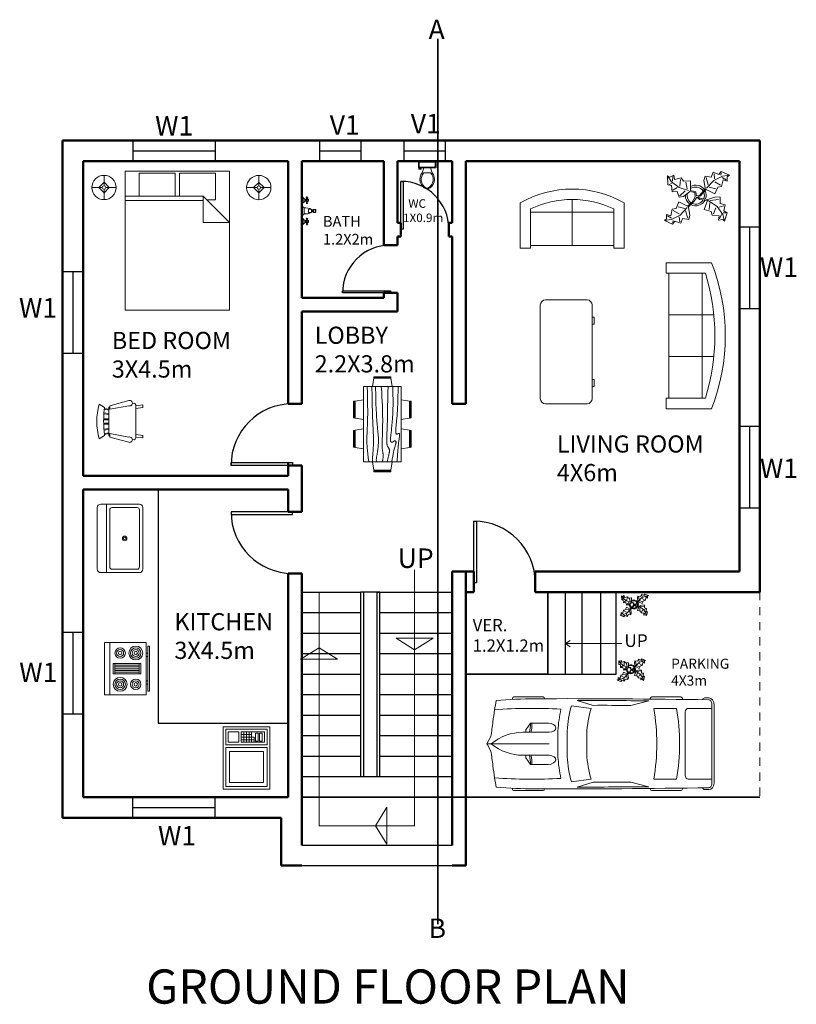
# Paper-space layout 'Layout1' of a CAD drawing. Units: metres. Extents: x 221.2 to 255.5, y 284.4 to 307.4.
# Tile 1 of 3: x 222.2 to 233.6, y 284.4 to 298.8. Entities that reach past the tile are written whole.
import ezdxf

# ---------------------------------------------------------------- set-up
doc = ezdxf.new("R2010")
doc.units = ezdxf.units.M
doc.linetypes.add('ACAD_ISO02W100', pattern=[15, 12, -3])
for name, color, linetype, lineweight in [('A-ANNO-SYMB', 1, 'Continuous', 18), ('A-AREA-IDEN', 11, 'Continuous', 25), ('A-EQPM', 20, 'Continuous', 18), ('A-FLOR-CASE', 20, 'Continuous', 25), ('A-FLOR-FIXT', 20, 'Continuous', 18), ('A-FLOR-PROJ', 7, 'ACAD_ISO02W100', 18), ('A-MODL', 7, 'Continuous', 25), ('A-WALL', 7, 'Continuous', 50), ('car', 150, 'Continuous', 18), ('door', 6, 'Continuous', 25), ('floor', 7, 'Continuous', 35), ('flower', 70, 'Continuous', 18), ('furnitures', 20, 'Continuous', 18), ('section', 1, 'Continuous', 35), ('stair', 2, 'Continuous', 25), ('text', 11, 'Continuous', 25), ('window', 3, 'Continuous', 25)]:
    doc.layers.add(name, color=color, linetype=linetype, lineweight=lineweight)
doc.styles.get("Standard").update_dxf_attribs({"font": 'arial.ttf'})

# ---------------------------------------------------------------- blocks, each defined once
blk = doc.blocks.new('*U21')
for p, q in [((0, 0), (0, -6)), ((40, 0), (40, -6))]:
    blk.add_line(p, q)
blk.add_lwpolyline([(0, 0), (0, 40), (1.75, 40), (1.75, 0)], close=True)
blk.add_arc((0, 0), 40, 0, 90)
blk = doc.blocks.new('*U2')
for p, q in [((0, 0), (0, -6)), ((-40, 0), (-40, -6))]:
    blk.add_line(p, q)
blk.add_lwpolyline([(0, 0), (0, 40), (-1.75, 40), (-1.75, 0)], close=True)
blk.add_arc((0, 0), 40, 90, 180)
blk = doc.blocks.new('Bed - Queen')
for p, q in [((0, -80.00003), (0, 0)), ((0, 0), (59.99999, 0)), ((59.99999, 0), (59.99999, -80.00003)), ((7.99999, -1.2), (28.79998, -1.2)), ((7.99999, -14.4), (7.99999, -1.2)), ((28.79998, -1.2), (28.79998, -14.4)), ((31.19999, -1.2), (51.99999, -1.2)), ((31.19999, -14.4), (31.19999, -1.2)), ((51.99999, -1.2), (51.99999, -16.4)), ((0, -14.4), (44.8, -14.4)), ((44.8, -16.8), (0, -16.8)), ((59.99999, -29.6), (44.8, -14.4)), ((44.8, -14.4), (44.8, -29.6)), ((51.99999, -16.4), (46.79936, -16.4)), ((44.8, -29.6), (59.99999, -29.6)), ((59.99999, -80.00003), (0, -80.00003))]:
    blk.add_line(p, q)
blk = doc.blocks.new('Chair - Rocking')
for p, q in [((-8, -4.5), (-10, -1.5)), ((-7.5, -4.5), (-7, -7)), ((-6.5, -7), (-7.02225, -4.43)), ((-4.5, -7), (-4.96674, -4.19951)), ((-4, -7), (-4.40532, -4.16272)), ((-1.5, -4.05012), (-1.5, -7)), ((-1, -7), (-1, -4.05012)), ((1, -7), (1, -4.04655)), ((1.5, -4.05012), (1.5, -7)), ((4, -7), (4.40187, -4.18694)), ((4.5, -7), (4.96761, -4.19437)), ((6.5, -7), (7, -4.4057)), ((7.5, -4.5), (7, -7)), ((8, -4.5), (10, -1.5)), ((-9, -7.5), (-12, -18.49999)), ((-7, -7.5), (-9, -7.5)), ((-9, -18.49999), (-7, -7.5)), ((-8.23428, -6.99939), (-8.3093, -7.47958)), ((-8.23041, -7), (8.23915, -7)), ((7, -7.5), (9, -7.5)), ((9, -18.49999), (7, -7.5)), ((8.31071, -7.48854), (8.23449, -7.00073)), ((9, -7.5), (12, -18.49999)), ((-10.36644, -20.64523), (-10.5, -21.49999)), ((-9, -22.49999), (-9.5, -26.49999)), ((0, -22.49999), (-9.5, -22.49999)), ((-8, -26.49999), (-7.5, -22.49999)), ((0, -22.49999), (9.5, -22.49999)), ((8, -26.49999), (7.5, -22.49999)), ((9, -22.49999), (9.5, -26.49999)), ((10.5, -21.49999), (10.3575, -20.58798)), ((-9.5, -26.49999), (-8, -26.49999)), ((9.5, -26.49999), (8, -26.49999))]:
    blk.add_line(p, q)
for centre, radius, start, end in [((0, -34.08333), 34.08333, 72.93847, 107.0615), ((0, -68.25004), 64.25, 93.92211, 97.15267), ((0, -68.25004), 64.25, 82.84733, 93.92211), ((-10.5, -18.99999), 1.58114, 161.5651, 18.43495), ((-9.5, -21.49999), 1, 180, 270), ((10.5, -18.99999), 1.58114, 161.5651, 18.43495), ((9.5, -21.49999), 1, 270, 0)]:
    blk.add_arc(centre, radius, start, end)
blk = doc.blocks.new('Dining Set - 36 x 72 in.')
for p, q in [((-22.2343, 26.00059), (-23.4847, 17.99762)), ((-22.2304, 26), (-5.7608, 26)), ((-22, 27.5), (-22.1562, 26.50042)), ((-5.8416, 26.5), (-22.1534, 26.5)), ((-22, 27.5), (-6, 27.5)), ((-5.8437, 26.49966), (-6, 27.5)), ((-4.5152, 17.99762), (-5.7655, 25.99926)), ((5.7657, 26.00059), (4.5153, 17.99762)), ((5.7696, 26), (22.2392, 26)), ((6, 27.5), (5.8438, 26.50042)), ((22.1584, 26.5), (5.8466, 26.5)), ((6, 27.5), (22, 27.5)), ((22.1563, 26.49966), (22, 27.5)), ((23.4848, 17.99762), (22.2345, 25.99926)), ((-44.0006, 8.23428), (-35.9976, 9.48474)), ((36, 18), (-36, 18)), ((-36, 18), (-36, -18)), ((44.0006, 8.23428), (35.9976, 9.48474)), ((36, -18), (36, 18)), ((-45.5, 8), (-44.5004, 8.15617)), ((-45.5, 8), (-45.5, -8)), ((-44.5, -8.15843), (-44.5, 8.15338)), ((-44, 8.23041), (-44, -8.23915)), ((44, 8.23041), (44, -8.23915)), ((44.5, -8.15843), (44.5, 8.15338)), ((45.5, 8), (44.5005, 8.15617)), ((45.5, 8), (45.5, -8)), ((-44.4997, -8.15631), (-45.5, -8)), ((-35.9976, -9.48476), (-43.9993, -8.2345)), ((35.9976, -9.48476), (43.9993, -8.2345)), ((44.4997, -8.15631), (45.5, -8)), ((-36, -18), (36, -18)), ((-22.2343, -26.0006), (-23.4847, -17.99762)), ((-4.5152, -17.99762), (-5.7655, -25.99928)), ((5.7657, -26.0006), (4.5153, -17.99762)), ((23.4848, -17.99762), (22.2345, -25.99928)), ((-22.2304, -26), (-5.7608, -26)), ((-22, -27.5), (-22.1562, -26.50044)), ((-5.8416, -26.5), (-22.1534, -26.5)), ((-22, -27.5), (-6, -27.5)), ((-5.8437, -26.49967), (-6, -27.5)), ((5.7696, -26), (22.2392, -26)), ((6, -27.5), (5.8438, -26.50044)), ((22.1584, -26.5), (5.8466, -26.5)), ((6, -27.5), (22, -27.5)), ((22.1563, -26.49967), (22, -27.5))]:
    blk.add_line(p, q)
for points in [[(-36, 15), (-31.1772, 14.97754), (-26.8079, 14.91406), (-22.8538, 14.81543), (-19.276, 14.6875), (-16.0362, 14.53613), (-13.0957, 14.36718), (-10.4159, 14.18652), (-7.9583, 14), (-5.6904, 13.81315), (-3.6035, 13.63021), (-1.6954, 13.45508), (0.0365, 13.29166), (1.5945, 13.14388), (2.9811, 13.01562), (4.1988, 12.9108), (5.25, 12.83333), (6.1393, 12.78613), (6.8802, 12.76823), (7.4883, 12.77767), (7.9792, 12.8125), (8.3685, 12.87077), (8.6719, 12.95052), (8.9049, 13.0498), (9.0833, 13.16666), (9.2205, 13.29899), (9.3216, 13.44401), (9.3895, 13.59879), (9.4271, 13.76041), (9.4373, 13.92594), (9.4232, 14.09245), (9.3875, 14.257), (9.3333, 14.41666), (9.2638, 14.56917), (9.1836, 14.71484), (9.0975, 14.85465), (9.0104, 14.98958), (8.9272, 15.1206), (8.8529, 15.2487), (8.7922, 15.37483), (8.75, 15.5), (8.7305, 15.62467), (8.7344, 15.74739), (8.7617, 15.86621), (8.8125, 15.97916), (8.8867, 16.08431), (8.9844, 16.17968), (9.1055, 16.26334), (9.25, 16.33333), (9.4189, 16.38802), (9.6172, 16.42708), (9.8506, 16.45052), (10.125, 16.45833), (10.4463, 16.45052), (10.8203, 16.42708), (11.2529, 16.38802), (11.75, 16.33333), (12.3184, 16.26318), (12.9694, 16.17838), (13.7151, 16.07991), (14.5677, 15.96875), (15.5395, 15.84586), (16.6426, 15.71224), (17.8893, 15.56884), (19.2917, 15.41666), (20.859, 15.25667), (22.5879, 15.08984), (24.4721, 14.91715), (26.5052, 14.73958), (28.6809, 14.5581), (30.9929, 14.3737), (33.4347, 14.18733), (36, 14)], [(-36, 10), (-28.9766, 10.14274), (-23.1725, 10.20442), (-18.4241, 10.19775), (-14.5677, 10.13541), (-11.4399, 10.03011), (-8.877, 9.89453), (-6.7154, 9.74137), (-4.7917, 9.58333), (-2.9698, 9.43082), (-1.2246, 9.28515), (0.4415, 9.14534), (2.026, 9.01041), (3.5266, 8.87939), (4.9408, 8.7513), (6.266, 8.62516), (7.5, 8.5), (8.6411, 8.37549), (9.6914, 8.2539), (10.6538, 8.13818), (11.5312, 8.03125), (12.3267, 7.93603), (13.043, 7.85547), (13.6831, 7.79248), (14.25, 7.75), (14.7471, 7.7303), (15.1797, 7.73307), (15.5537, 7.75732), (15.875, 7.80208), (16.1494, 7.86637), (16.3828, 7.94922), (16.5811, 8.04964), (16.75, 8.16666), (16.8944, 8.29915), (17.0143, 8.44531), (17.1089, 8.60319), (17.1771, 8.77083), (17.218, 8.94629), (17.2305, 9.1276), (17.2137, 9.31282), (17.1667, 9.5), (17.0895, 9.6875), (16.987, 9.875), (16.8649, 10.0625), (16.7292, 10.25), (16.5856, 10.4375), (16.4401, 10.625), (16.2985, 10.8125), (16.1667, 11), (16.05, 11.18733), (15.9518, 11.3737), (15.8752, 11.5581), (15.8229, 11.73958), (15.798, 11.91715), (15.8034, 12.08984), (15.842, 12.25667), (15.9167, 12.41666), (16.0295, 12.56836), (16.1784, 12.70833), (16.3605, 12.83268), (16.5729, 12.9375), (16.8127, 13.01888), (17.0768, 13.07291), (17.3625, 13.0957), (17.6667, 13.08333), (17.9894, 13.03312), (18.3418, 12.94726), (18.7382, 12.82918), (19.1927, 12.68229), (19.7195, 12.51001), (20.3327, 12.31575), (21.0465, 12.10294), (21.875, 11.875), (22.8357, 11.63354), (23.959, 11.37304), (25.2786, 11.08618), (26.8282, 10.76562), (28.6414, 10.40405), (30.752, 9.99414), (33.1936, 9.52856), (36, 9)], [(-36, 5.5), (-30.7157, 5.3348), (-26.069, 5.20963), (-21.9946, 5.11767), (-18.4271, 5.05208), (-15.3009, 5.00602), (-12.5508, 4.97265), (-10.1112, 4.94515), (-7.9167, 4.91666), (-5.909, 4.88167), (-4.0586, 4.83984), (-2.3429, 4.79215), (-0.7396, 4.73958), (0.7739, 4.6831), (2.22, 4.6237), (3.6213, 4.56233), (5, 4.5), (6.373, 4.43782), (7.7344, 4.3776), (9.0723, 4.32129), (10.375, 4.27083), (11.6309, 4.22819), (12.8281, 4.19531), (13.9551, 4.17415), (15, 4.16666), (15.954, 4.17448), (16.819, 4.19791), (17.6001, 4.23698), (18.3021, 4.29166), (18.9299, 4.36198), (19.4883, 4.44791), (19.9823, 4.54948), (20.4167, 4.66666), (20.7969, 4.79899), (21.1302, 4.94401), (21.4245, 5.09879), (21.6875, 5.26041), (21.9271, 5.42594), (22.1511, 5.59245), (22.3672, 5.757), (22.5834, 5.91666), (22.8065, 6.06868), (23.0404, 6.21093), (23.2879, 6.34147), (23.5521, 6.45833), (23.8358, 6.55957), (24.142, 6.64323), (24.4735, 6.70735), (24.8334, 6.75), (25.2235, 6.76969), (25.642, 6.76692), (26.0858, 6.74267), (26.5521, 6.69791), (27.0379, 6.63362), (27.5404, 6.55078), (28.0565, 6.45036), (28.5834, 6.33333), (29.1242, 6.19987), (29.7071, 6.04687), (30.3661, 5.87044), (31.1354, 5.66666), (32.0493, 5.43164), (33.142, 5.16146), (34.4475, 4.85221), (36, 4.5)], [(-36, -1), (-30.7915, -0.6591), (-26.0195, -0.38216), (-21.6519, -0.16284), (-17.6563, 0.00521), (-14.0005, 0.12833), (-10.6523, 0.21289), (-7.5796, 0.26522), (-4.75, 0.29166), (-2.134, 0.29793), (0.2878, 0.28711), (2.5317, 0.26163), (4.6146, 0.22396), (6.5529, 0.17651), (8.3633, 0.12174), (10.0623, 0.06209), (11.6667, 0), (13.1899, -0.06201), (14.6341, -0.1211), (15.9982, -0.17432), (17.2813, -0.21875), (18.4823, -0.25147), (19.6003, -0.26953), (20.6343, -0.27002), (21.5834, -0.25), (22.4481, -0.20768), (23.2357, -0.14584), (23.9549, -0.06836), (24.6146, 0.02083), (25.2235, 0.11784), (25.7904, 0.21875), (26.3241, 0.31966), (26.8334, 0.41666), (27.3265, 0.50618), (27.8099, 0.58593), (28.2894, 0.65397), (28.7709, 0.70833), (29.2601, 0.74707), (29.763, 0.76823), (30.2855, 0.76985), (30.8334, 0.75), (31.4088, 0.70784), (31.9994, 0.64713), (32.589, 0.57275), (33.1615, 0.48958), (33.7008, 0.4025), (34.1908, 0.3164), (34.6153, 0.23616), (34.9584, 0.16666), (35.2099, 0.11165), (35.3848, 0.07031), (35.504, 0.04069), (35.5886, 0.02083), (35.6594, 0.00879), (35.7377, 0.0026), (35.8442, 0.00032), (36, 0)], [(-36, -6.5), (-27.1843, -6.31267), (-20.084, -6.1263), (-14.469, -5.9419), (-10.1094, -5.76042), (-6.7752, -5.58285), (-4.2363, -5.41016), (-2.2629, -5.24333), (-0.625, -5.08334), (0.8708, -4.93099), (2.2715, -4.78646), (3.5872, -4.64974), (4.8281, -4.52084), (6.0046, -4.39974), (7.127, -4.28646), (8.2053, -4.18099), (9.25, -4.08334), (10.2705, -3.99382), (11.2734, -3.91407), (12.2647, -3.84603), (13.25, -3.79167), (14.2354, -3.75293), (15.2266, -3.73177), (16.2295, -3.73015), (17.25, -3.75), (18.2912, -3.79248), (19.3451, -3.85547), (20.4009, -3.93604), (21.4479, -4.03125), (22.4754, -4.13819), (23.4727, -4.25391), (24.4289, -4.37549), (25.3334, -4.5), (26.1785, -4.62492), (26.9694, -4.74935), (27.7145, -4.87281), (28.4219, -4.99479), (29.1, -5.11483), (29.7572, -5.23242), (30.4016, -5.34709), (31.0417, -5.45834), (31.6837, -5.56437), (32.3262, -5.65821), (32.9658, -5.73153), (33.599, -5.77604), (34.2224, -5.78345), (34.8327, -5.74545), (35.4264, -5.65373), (36, -5.5)], [(-36, -10), (-26.4022, -9.81299), (-18.4675, -9.62891), (-11.9839, -9.45069), (-6.7396, -9.28125), (-2.5226, -9.12354), (0.8789, -8.98047), (3.6769, -8.85498), (6.0833, -8.75), (8.2767, -8.66765), (10.3021, -8.60677), (12.1712, -8.56543), (13.8958, -8.54167), (15.4876, -8.53353), (16.9583, -8.53907), (18.3197, -8.55632), (19.5834, -8.58334), (20.7616, -8.61841), (21.8685, -8.66081), (22.9188, -8.71004), (23.9271, -8.76563), (24.9081, -8.82707), (25.8763, -8.89388), (26.8465, -8.96558), (27.8334, -9.04167), (28.8474, -9.12118), (29.8828, -9.20117), (30.93, -9.27824), (31.9792, -9.34896), (33.0205, -9.40991), (34.0443, -9.45768), (35.0407, -9.48885), (36, -9.5)], [(-36, -14.5), (-30.0881, -14.33513), (-25.0332, -14.21224), (-20.7312, -14.12647), (-17.0781, -14.07292), (-13.97, -14.04671), (-11.3027, -14.04297), (-8.9724, -14.05681), (-6.875, -14.08334), (-4.9224, -14.11833), (-3.0905, -14.16016), (-1.3709, -14.20785), (0.2448, -14.26042), (1.7647, -14.3169), (3.1973, -14.3763), (4.5507, -14.43767), (5.8333, -14.5), (7.0554, -14.5621), (8.235, -14.62175), (9.3922, -14.67652), (10.5469, -14.72396), (11.7192, -14.76164), (12.929, -14.78711), (14.1965, -14.79794), (15.5417, -14.79167), (16.9933, -14.76424), (18.6152, -14.70508), (20.4804, -14.60197), (22.6615, -14.44271), (25.2312, -14.21509), (28.2624, -13.9069), (31.8277, -13.50594), (36, -13)]]:
    blk.add_lwpolyline(points)
blk = doc.blocks.new('Plant - Rubber or Philodendron')
for p, q in [((-16.2005, 11.4774), (-13.9899, 8.1064)), ((-16.2005, 11.4774), (-14.8639, 10.7964)), ((-16.0159, 6.3329), (-16.2005, 11.4774)), ((-14.8639, 10.7964), (-12.6195, 11.8975)), ((-12.6195, 11.8975), (-12.1909, 9.4345)), ((8.8871, 10.7908), (9.9809, 13.4933)), ((9.9809, 13.4933), (13.3837, 12.301)), ((10.5828, 12.6946), (10.8893, 9.7953)), ((13.3837, 12.301), (14.68, 13.9039)), ((14.5816, 13.2037), (14.3848, 11.8033)), ((14.68, 13.9039), (19.3848, 11.8146)), ((19.3848, 11.8146), (15.3859, 11.3055)), ((19.3848, 11.8146), (18.1868, 10.9119)), ((-14.0069, 5.8704), (-16.0159, 6.3329)), ((-15.3434, 6.5514), (-13.9984, 6.9884)), ((-13.5868, 2.2894), (-14.0069, 5.8704)), ((-13.9899, 8.1064), (-9.5434, 4.7185)), ((-13.3174, 8.325), (-13.0735, 11.0065)), ((-12.1909, 9.4345), (-8.3829, 10.3)), ((-8.8369, 9.409), (-9.0894, 5.6095)), ((-8.3829, 10.3), (-7.0549, 8.501)), ((-7.0549, 8.501), (-3.0284, 8.6941)), ((-4.8529, 4.012), (-5.7184, 7.82)), ((-3.0284, 8.6941), (-3.0709, 3.1041)), ((4.6914, 8.8812), (5.3859, 11.2828)), ((4.6914, 8.8812), (5.5014, 4.4831)), ((5.3859, 11.2828), (8.8871, 10.7908)), ((5.9878, 10.4842), (7.1971, 6.3869)), ((10.3916, 8.7942), (6.2847, 4.4028)), ((15.3859, 11.3055), (10.3916, 8.7942)), ((14.2977, 6.1031), (10.9934, 7.9956)), ((15.7909, 9.1065), (14.8995, 5.3044)), ((15.2875, 10.6053), (17.5907, 9.2105)), ((18.1925, 8.4119), (15.7909, 9.1065)), ((18.1868, 10.9119), (18.1925, 8.4119)), ((-10.6784, 2.491), (-13.5868, 2.2894)), ((-13.1329, 3.1804), (-10.6614, 4.727)), ((-9.5858, -0.8715), (-10.6784, 2.491)), ((-9.5434, 4.7185), (-4.1917, 2.9888)), ((-9.1318, 0.0195), (-5.9793, 2.9025)), ((-7.1228, -0.443), (-3.5248, 2.2131)), ((-3.5248, 2.2131), (-3.3011, 2.4355)), ((-3.3011, 2.4355), (-0.5306, 1.7947)), ((-3.0709, 3.1041), (0.0797, 2.3163)), ((-0.5306, 1.7947), (-0.2255, -0.5527)), ((-0.5306, 1.7947), (-0.5306, 1.7947)), ((0.0797, 2.3163), (0.4866, -0.031)), ((0.4866, -0.031), (2.1141, 0.2298)), ((2.1141, 0.2298), (5.4346, 3.9146)), ((6.1032, 3.6844), (2.8262, -0.031)), ((5.4346, 3.9146), (5.5014, 4.4831)), ((11.1089, 1.1958), (6.1032, 3.6844)), ((7.7005, 4.8881), (11.5025, 3.9967)), ((12.7005, 4.8994), (11.1089, 1.1958)), ((14.8995, 5.3044), (12.7005, 4.8994)), ((-11.3237, -7.2629), (-9.7321, -3.5593)), ((-9.7321, -3.5593), (-4.7264, -6.0479)), ((-7.1228, -0.443), (-9.5858, -0.8715)), ((-2.019, -3.6148), (-4.7264, -6.0479)), ((-4.0579, -6.2781), (-0.9375, -3.1608)), ((-2.019, -3.6148), (-0.2255, -0.5527)), ((-0.9375, -3.1608), (0.5883, -0.8135)), ((0.5883, -0.8135), (2.2447, -2.0916)), ((2.8262, -0.031), (1.3003, -0.5527)), ((1.3003, -0.5527), (2.4193, -1.4655)), ((2.2447, -2.0916), (6.7108, -2.6626)), ((2.4193, -1.4655), (6.895, -2.1175)), ((4.943, -7.9659), (6.7108, -2.6626)), ((11.6605, -0.5413), (6.895, -2.1175)), ((12.3677, -6.1981), (7.219, -2.6772)), ((8.125, -4.0768), (7.7715, -7.9659)), ((8.3544, -2.7453), (13.1973, -2.1704)), ((11.6605, -0.5413), (14.1354, -0.8948)), ((14.1354, -0.8948), (14.1354, -4.4304)), ((14.1354, -4.4304), (16.9638, -5.1375)), ((16.9638, -5.1375), (16.2567, -8.673)), ((-16.8157, -10.7754), (-14.4141, -11.4699)), ((-16.8101, -13.2754), (-16.8157, -10.7754)), ((-14.4141, -11.4699), (-13.5228, -7.6679)), ((-14.0091, -13.669), (-9.0148, -11.1577)), ((-13.5228, -7.6679), (-11.3237, -7.2629)), ((-12.921, -8.4665), (-9.6166, -10.359)), ((-6.3237, -7.2516), (-10.1257, -6.3602)), ((-9.0148, -11.1577), (-4.9047, -6.8122)), ((-4.611, -12.8477), (-5.8203, -8.7504)), ((-4.1246, -6.8466), (-4.0579, -6.2781)), ((-3.3146, -11.2447), (-4.1246, -6.8466)), ((-3.3146, -11.2447), (-4.0092, -13.6463)), ((8.8321, -9.0266), (4.943, -7.9659)), ((9.5392, -11.1479), (8.8321, -9.0266)), ((13.4283, -11.5015), (9.5392, -11.1479)), ((10.2463, -10.4408), (11.6605, -6.9053)), ((15.5496, -10.7943), (12.3677, -6.1981)), ((16.2567, -5.8446), (13.4283, -6.5517)), ((14.8425, -10.7943), (13.7819, -13.2692)), ((16.6103, -14.6834), (15.5496, -10.7943)), ((17.3174, -9.7337), (15.9032, -9.7337)), ((16.2567, -8.673), (18.0245, -9.7337)), ((18.0245, -9.7337), (16.6103, -14.6834)), ((-18.008, -14.1781), (-16.8101, -13.2754)), ((-18.008, -14.1781), (-14.0091, -13.669)), ((-13.3032, -16.2674), (-18.008, -14.1781)), ((-13.9107, -12.9688), (-16.2139, -11.574)), ((-12.0069, -14.6645), (-13.3032, -16.2674)), ((-13.2048, -15.5672), (-13.008, -14.1668)), ((-8.6042, -15.8568), (-12.0069, -14.6645)), ((-9.206, -15.0581), (-9.5126, -12.1588)), ((-7.5103, -13.1543), (-8.6042, -15.8568)), ((-4.0092, -13.6463), (-7.5103, -13.1543)), ((13.0748, -13.9763), (13.4283, -11.5015)), ((15.5496, -13.6228), (13.0748, -13.9763)), ((16.6103, -14.6834), (15.5496, -13.6228))]:
    blk.add_line(p, q)
for centre, radius, start, end in [((0, 0), 6.1275, 34.37569, 120.1028), ((0.0308, 0.1664), 6, 178.6147, 235.1169), ((0.0308, 0.1664), 5, 168.1647, 238.6725), ((-0.0601, -0.2075), 5.2461, 33.82192, 124.9414), ((-0.2664, 0.1682), 5.2775, 338.4094, 20.03007), ((-0.098, 0.1364), 6.1288, 341.2017, 26.09184), ((-0.0234, 0.3825), 6.1492, 242.5812, 331.2714), ((-0.1102, 0.4886), 5.2883, 247.3711, 327.472)]:
    blk.add_arc(centre, radius, start, end)
blk = doc.blocks.new('Sofa - Roundback 7 ft.')
for p, q in [((-12.00002, -32.4421), (-12.00003, -6.5971)), ((11.99997, -32.4421), (11.99998, -6.5971)), ((-36.000027, -34), (-36.000027, -11.4696)), ((-35.999844, -13.3819), (35.9998, -13.3819)), ((35.99998, -34), (35.99998, -11.4696)), ((-36.000027, -32.4421), (35.99998, -32.4421))]:
    blk.add_line(p, q)
for points in [[(-36.000027, -34), (-42.000027, -34), (-42.000027, -8)], [(41.99998, -8), (41.99998, -34), (35.99998, -34)]]:
    blk.add_lwpolyline(points)
for centre, radius, start, end in [((0, -114.25), 114.25, 68.43141, 111.5686), ((-0.00001, -127.1968), 121.1968, 72.72033, 107.2797)]:
    blk.add_arc(centre, radius, start, end)
blk = doc.blocks.new('Sofa - Roundback Loveseat 5 ft.')
for p, q in [((0, -32.44198), (0, -5.99998)), ((-24, -33.99998), (-24, -11.46958)), ((-23.9998, -13.38178), (23.99986, -13.38178)), ((24.00004, -33.99998), (24.00004, -11.46958)), ((-24, -32.44198), (24.00004, -32.44198))]:
    blk.add_line(p, q)
for points in [[(-24, -33.99998), (-30, -33.99998), (-30, -7.99998)], [(30.00004, -7.99998), (30.00004, -33.99998), (24.00004, -33.99998)]]:
    blk.add_lwpolyline(points)
for centre, radius, start, end in [((0, -60.24998), 60.24998, 60.13715, 119.8628), ((0, -61.38438), 55.38444, 64.32083, 115.6792)]:
    blk.add_arc(centre, radius, start, end)
blk = doc.blocks.new('Desk - 30 x 60 in.')
for p, q in [((-26.999995, 0), (26.999995, 0)), ((-29.999995, -27), (-29.999995, -3)), ((29.999995, -3), (29.999995, -27)), ((26.999995, -30), (-26.999995, -30)), ((-20.000005, -30), (-20.000005, -31)), ((-20.000005, -31), (-16.000005, -31)), ((-16.000005, -31), (-16.000005, -30)), ((15.999995, -31), (15.999995, -30)), ((19.999995, -31), (15.999995, -31)), ((19.999995, -30), (19.999995, -31))]:
    blk.add_line(p, q)
for centre, start, end in [((-26.499995, -3.5), 98.1301, 171.8699), ((26.499995, -3.5), 8.130102, 81.8699), ((-26.499995, -26.5), 188.1301, 261.8699), ((26.499995, -26.5), 278.1301, 351.8699)]:
    blk.add_arc(centre, 3.535534, start, end)
blk = doc.blocks.new('Microwave')
for p, q in [((18, 10), (22, 10)), ((22, 9), (18, 9)), ((18, 8), (22, 8)), ((19, 7), (19, 11)), ((20, 11), (20, 7)), ((21, 7), (21, 11)), ((22, 7), (18, 7)), ((20, 6), (18, 6)), ((19, 6), (19, 7)), ((20, 7), (20, 6))]:
    blk.add_line(p, q)
for points in [[(0, 0), (0, 18), (24, 18), (24, 0)], [(1, 1), (1, 17), (16, 17), (16, 1)], [(2.5, 2.5), (2.5, 15.5), (14.5, 15.5), (14.5, 2.5)], [(17, 1), (17, 17), (23, 17), (23, 1)], [(18, 12), (18, 16), (22, 16), (22, 12)], [(18, 2), (18, 11), (22, 11), (22, 2)], [(18.5, 4.5), (18.5, 5.5), (21.5, 5.5), (21.5, 4.5)], [(18.5, 3), (18.5, 4), (21.5, 4), (21.5, 3)]]:
    blk.add_lwpolyline(points, close=True)
blk = doc.blocks.new('Range-Oven - 30 in top')
for p, q in [((0, -3), (30, -3)), ((12, -6), (18, -6)), ((13, -20), (13, -6)), ((14, -6), (14, -20)), ((15, -20), (15, -6)), ((16, -6), (16, -20)), ((17, -20), (17, -6)), ((18, -20), (12, -20)), ((6, -24), (6, -25)), ((8, -25), (8, -24)), ((22, -25), (22, -24)), ((24, -24), (24, -25))]:
    blk.add_line(p, q)
for points in [[(0, -24), (0, 0), (30, 0), (30, -24)], [(12, -21), (12, -5), (18, -5), (18, -21)], [(2, -26), (2, -25), (28, -25), (28, -26)]]:
    blk.add_lwpolyline(points, close=True)
for centre, radius in [((6, -9), 4), ((6, -9), 3), ((6, -9), 2), ((6, -9), 1), ((24, -9), 3), ((24, -9), 2), ((24, -9), 1), ((6, -18), 3), ((6, -18), 2), ((6, -18), 1), ((24, -18), 4), ((24, -18), 3), ((24, -18), 2), ((24, -18), 1)]:
    blk.add_circle(centre, radius)
blk = doc.blocks.new('Sink-single - 30 in top')
blk.add_line((-15, -3.999996), (15, -3.999996))
for points in [[(-13.5, 0), (13.5, 0)], [(-15, -18.499996), (-15, -1.5)], [(15, -1.5), (15, -18.499996)], [(-13.5, -17.499996), (-13.5, -6.499996)], [(-12.5, -5.499996), (12.5, -5.499996)], [(13.5, -6.499996), (13.5, -17.499996)], [(13.5, -19.999996), (-13.5, -19.999996)], [(12.5, -18.499996), (-12.5, -18.499996)]]:
    blk.add_lwpolyline(points)
for radius in [1, 0.5]:
    blk.add_circle((0, -11.999996), radius)
for centre, radius, start, end in [((-13.5, -1.5), 1.5, 90, 180), ((13.5, -1.5), 1.5, 0, 90), ((-12.5, -6.499996), 1, 90, 180), ((12.5, -6.499996), 1, 0, 90), ((-13.5, -18.499996), 1.5, 180, 270), ((-12.5, -17.499996), 1, 180, 270), ((12.5, -17.499996), 1, 270, 0), ((13.5, -18.499996), 1.5, 270, 0)]:
    blk.add_arc(centre, radius, start, end)
blk = doc.blocks.new('Lamp - Table')
for p, q in [((0, 7), (0, 1)), ((-1, 0), (-7, 0)), ((0, 3), (-3, 0)), ((-3, 0), (0, -3)), ((3, 0), (0, 3)), ((0, -3), (3, 0)), ((1, 0), (7, 0)), ((0, -1), (0, -7))]:
    blk.add_line(p, q)
for radius in [7, 1]:
    blk.add_circle((0, 0), radius)
blk = doc.blocks.new('Toilet - top')
for p, q in [((-10, -8.5), (-8, -8.5)), ((-10, -9.5), (-10, -8.5)), ((-7, -9.5), (-10, -9.5)), ((-8, -8.5), (-8, -8)), ((-7, -8), (-7, -9.5)), ((-4, -8), (-6, -14)), ((4, -8), (6, -14)), ((9.5, -6), (9.5, -2)), ((4, -14), (-4, -14))]:
    blk.add_line(p, q)
blk.add_lwpolyline([(10.5, -8), (10.5, 0), (-10.5, 0), (-10.5, -8)], close=True)
for points in [[(-9.5, -2), (-9.5, -6)], [(8.5, -1), (-8.5, -1)], [(-8.5, -7), (8.5, -7)]]:
    blk.add_lwpolyline(points)
for centre, radius, start, end in [((-8.6, -1.9), 0.884, 81.8699, 188.1301), ((-8.6, -6.1), 0.884, 171.8699, 278.1301), ((8.6, -1.9), 0.884, 351.8699, 98.1301), ((8.6, -6.1), 0.884, 261.8699, 8.1301), ((3.5, -21.6), 12.2, 141.4691, 247.9714), ((4.2, -21.8), 11.3, 136.3677, 238.9468), ((-3.5, -21.6), 12.2, 292.0284, 38.5307), ((-4.2, -21.8), 11.3, 301.053, 43.6321), ((0, -27.9), 4, 245.7318, 294.2682), ((0, -29), 4, 254.8605, 285.1395)]:
    blk.add_arc(centre, radius, start, end)
blk = doc.blocks.new('Faucet - Bathroom front')
for p, q in [((-0.5, 4.25), (0.5, 4.25)), ((0.5, 3.75), (-0.5, 3.75)), ((-0.25, 3), (-0.25, 3.5)), ((0.25, 3.5), (0.25, 3)), ((-5, 0), (-2.25, 0)), ((-4.5087, 0.25), (-2.7408, 0.25)), ((-4, 1.625), (-4.25, 1.625)), ((-4, 1.375), (-4.25, 1.375)), ((-3.1442, 0.75), (-4.0979, 0.75)), ((-3.25, 1.625), (-3, 1.625)), ((-3.25, 1.375), (-3, 1.375)), ((-1.5, 0), (1.5, 0)), ((-1, 0.5), (1, 0.5)), ((-0.5, 3), (0.5, 3)), ((0.5, 2), (-0.5, 2)), ((2.25, 0), (5, 0)), ((2.7413, 0.25), (4.5092, 0.25)), ((3.25, 1.625), (3, 1.625)), ((3.25, 1.375), (3, 1.375)), ((4.1058, 0.75), (3.1521, 0.75)), ((4, 1.625), (4.25, 1.625)), ((4, 1.375), (4.25, 1.375))]:
    blk.add_line(p, q)
for points in [[(-0.5, 3.75), (-0.5, 4.25)], [(-0.25, 4.5), (0.25, 4.5)], [(0.25, 3.5), (-0.25, 3.5)], [(0.5, 4.25), (0.5, 3.75)]]:
    blk.add_lwpolyline(points)
for points in [[(-4, 1), (-4, 2), (-3.25, 2), (-3.25, 1)], [(3.25, 1), (3.25, 2), (4, 2), (4, 1)]]:
    blk.add_lwpolyline(points, close=True)
for centre in [(-4.5, 1.5), (-3.625, 1.5), (-2.75, 1.5), (2.75, 1.5), (3.625, 1.5), (4.5, 1.5)]:
    blk.add_circle(centre, 0.2795)
for centre, radius, start, end in [((-0.2575, 4.2575), 0.2426, 88.22243, 181.7776), ((-0.2575, 3.7425), 0.2426, 178.2224, 271.7776), ((0.2575, 4.2575), 0.2426, 358.2224, 91.77757), ((0.2575, 3.7425), 0.2426, 268.2224, 1.777565), ((-5.375, 1.375), 1.4252, 285.2551, 344.7449), ((-1.875, 1.375), 1.4252, 195.2551, 254.7449), ((-0.7962, -0.2038), 0.7327, 106.1502, 163.8498), ((3, 1), 4.0311, 150.2551, 187.125), ((0.6413, 2.5), 1.246, 156.3417, 203.6583), ((-3, 1), 4.0311, 352.875, 29.74488), ((-0.6413, 2.5), 1.246, 336.3417, 23.65835), ((0.7962, -0.2038), 0.7327, 16.1502, 73.84979), ((1.875, 1.375), 1.4252, 285.2551, 344.7449), ((5.375, 1.375), 1.4252, 195.2551, 254.7449)]:
    blk.add_arc(centre, radius, start, end)
blk = doc.blocks.new('*U17')
for p, q in [((21.1, 37.41), (21.1, 36.83)), ((46.55, 38.89), (22.35, 38.89)), ((47.8, 37.39), (47.8, 37.41)), ((87.99, 31.87), (74.76, 35.92)), ((134.31, 35.6), (119.29, 31.78)), ((135.45, 37.07), (135.45, 37.41)), ((136.7, 38.89), (160.9, 38.89)), ((162.15, 37.41), (162.15, 36.77)), ((186.47, -33.5), (186.47, 33.5)), ((188.4, -32.76), (188.4, 32.76)), ((70.03, 31.54), (86.41, 29.35)), ((138.42, 29.35), (157.25, 29.35)), ((164.52, 26.39), (164.52, -26.39)), ((186.47, 29.35), (167.01, 29.35)), ((32.27, 11.63), (36.13, 17.17)), ((36.13, 17.17), (50.94, 17.17)), ((29.77, 9.51), (51.68, 9.51)), ((32.12, 9.51), (32.12, 11.15)), ((58.92, -10.77), (58.92, 10.77)), ((66.55, -10.53), (66.55, 10.53)), ((82.74, 8.5), (82.74, -8.5)), ((186.47, -10.53), (186.47, 10.53)), ((3.27, 6.13), (0.1, 0.41)), ((0, 0), (51.68, 0)), ((0.1, -0.41), (3.27, -6.13)), ((29.77, -9.51), (51.68, -9.51)), ((32.12, -9.51), (32.12, -11.15)), ((32.27, -11.63), (36.13, -17.17)), ((36.13, -17.17), (50.94, -17.17)), ((86.41, -29.35), (70.03, -31.54)), ((87.99, -31.87), (74.76, -35.92)), ((134.31, -35.6), (119.29, -31.78)), ((157.25, -29.35), (138.42, -29.35)), ((167.01, -29.35), (186.47, -29.35)), ((21.1, -37.41), (21.1, -36.83)), ((46.55, -38.89), (22.35, -38.89)), ((47.8, -37.39), (47.8, -37.41)), ((135.45, -37.07), (135.45, -37.41)), ((136.7, -38.89), (160.9, -38.89)), ((162.15, -37.41), (162.15, -36.77))]:
    blk.add_line(p, q)
for centre, major_axis, ratio, start_param, end_param in [((266.03, -27.52), (0, 313.31), 0.842304, 1.367076, 1.39176), ((41.19, -490.86), (0, 528.23), 0.842304, 0.00281, 0.075598), ((22.35, 37.41), (0, -1.48), 0.842304, 3.141593, 4.712389), ((64.48, -10555.62), (0, 10593.03), 0.842304, -0.013397, 0.002797), ((46.55, 37.41), (0, 1.48), 0.842304, -1.570796, 0), ((64.48, -10555.62), (0, -10591.55), 0.842304, 3.133765, 3.140441), ((136.7, 37.41), (0, -1.48), 0.842304, 3.141593, 4.712389), ((160.9, 37.41), (0, 1.48), 0.842304, -1.570796, 0), ((180.63, 35.84), (0, 2.22), 0.842304, -0.013017, 1.249894), ((64.48, -10556.36), (0, 10595.31), 0.842304, -0.013397, -0.013017), ((183.98, 33.5), (0, -2.96), 0.842304, 1.570796, 3.128196), ((183.98, 32.76), (0, -5.25), 0.842304, 1.570796, 3.128196), ((259.18, -27.52), (0, -305.3), 0.842304, 4.528606, 4.561838), ((37.47, -593.96), (0, -623.33), 0.842304, 3.096046, 3.200911), ((134.4, 5.39), (0, -89.78), 0.842304, 4.449482, 4.652344), ((135.29, 5.39), (0, 81.77), 0.842304, 1.245306, 1.50788), ((149.6, 2.8), (0, -79.58), 0.842304, 4.372215, 4.640744), ((95.79, -3666.35), (0, -3698.24), 0.842304, 3.134049, 3.144098), ((17.08, 0), (0, 147.02), 0.842304, 4.511394, 4.913384), ((35.91, 0), (0, 147.02), 0.842304, 4.511394, 4.913384), ((167.01, 26.39), (0, 2.96), 0.842304, 0, 1.570796), ((-204.49, 52.4), (0, -250.96), 0.842304, 1.385369, 1.434372), ((13.04, 17.01), (0, 27.42), 0.842304, 4.435146, 4.718221), ((14.2, 17.01), (0, 27.42), 0.842304, 4.435146, 4.718221), ((50.79, 13.34), (6.34, -0.36), 0.603834, -1.395552, 1.581315), ((29.77, -46.66), (0, 56.17), 0.842304, 0, 0.590319), ((32.75, 11.15), (0, 0.74), 0.842304, 0.879714, 1.570796), ((0.62, 0), (0, -0.74), 0.842304, 4.131459, 5.293319), ((-204.49, -52.4), (0, 250.96), 0.842304, -1.434372, -1.385369), ((29.77, 46.66), (0, 56.17), 0.842304, 2.551274, 3.141593), ((32.75, -11.15), (0, -0.74), 0.842304, 4.712389, 5.403472), ((13.04, -17.01), (0, -27.42), 0.842304, 1.564964, 1.848039), ((14.2, -17.01), (0, -27.42), 0.842304, 1.564964, 1.848039), ((134.4, -5.39), (0, -89.78), 0.842304, -1.510751, -1.307889), ((135.29, -5.39), (0, -81.77), 0.842304, -1.50788, -1.245306), ((149.6, -2.8), (0, -79.58), 0.842304, -1.499151, -1.230623), ((259.18, 27.52), (0, 305.3), 0.842304, 1.721348, 1.754579), ((266.03, 27.52), (0, 313.31), 0.842304, 1.749832, 1.774517), ((37.47, 593.96), (0, -623.33), 0.842304, -0.059319, 0.045547), ((95.79, 3666.35), (0, -3698.24), 0.842304, -0.002505, 0.007544), ((167.01, -26.39), (0, -2.96), 0.842304, 4.712389, 6.283185), ((41.19, 490.86), (0, -528.23), 0.842304, -0.075598, -0.00281), ((22.35, -37.41), (0, 1.48), 0.842304, 1.570796, 3.141593), ((64.48, 10555.62), (0, 10593.03), 0.842304, 3.138796, 3.15499), ((46.55, -37.41), (0, -1.48), 0.842304, 0, 1.570796), ((64.48, 10555.62), (0, -10591.55), 0.842304, 0.001152, 0.007828), ((136.7, -37.41), (0, -1.48), 0.842304, -1.570796, 0), ((160.9, -37.41), (0, 1.48), 0.842304, 3.141593, 4.712389), ((180.63, -35.84), (0, -2.22), 0.842304, -1.249894, 0.013017), ((64.48, 10556.36), (0, 10595.31), 0.842304, 3.15461, 3.15499), ((183.98, -33.5), (0, 2.96), 0.842304, 3.15499, 4.712389), ((183.98, -32.76), (0, -5.25), 0.842304, 0.013397, 1.570796)]:
    blk.add_ellipse(centre, major_axis=major_axis, ratio=ratio, start_param=start_param, end_param=end_param)
at = {"extrusion": (0, 0, -1)}
blk.add_ellipse((50.79, -13.34), major_axis=(6.34, 0.36), ratio=0.603834, start_param=-1.395552, end_param=1.581315, dxfattribs=at)
blk = doc.blocks.new('aditya')
at = {"layer": 'A-ANNO-SYMB'}
for p, q in [((5.15, 3.623), (5.15, -0.117)), ((3.752, -0.117), (3.752, 3.3)), ((5.421, 2.623), (4.879, 2.623)), ((4.879, 2.623), (5.15, 2.457)), ((5.421, 2.623), (5.15, 2.457)), ((3.481, 2.316), (3.752, 2.482)), ((4.023, 2.316), (3.752, 2.482)), ((7.358, 2.546), (7.425, 2.591)), ((8.182, 2.546), (7.358, 2.546)), ((7.358, 2.546), (7.427, 2.498)), ((3.481, 2.316), (4.023, 2.316)), ((4.745, 0.154), (4.579, -0.117)), ((4.745, -0.388), (4.745, 0.154)), ((5.15, -0.117), (3.752, -0.117)), ((4.745, -0.388), (4.579, -0.117))]:
    blk.add_line(p, q, dxfattribs=at)
at = {"layer": 'A-FLOR-CASE'}
for points in [[(1.398, 0.3), (0.3, 0.3), (0.3, 4.8), (1.398, 4.8), (1.398, 1.383)], [(1.398, 1.383), (3.3, 1.383), (3.3, 0.3), (0.3, 0.3), (0.3, 1.383)]]:
    blk.add_lwpolyline(points, dxfattribs=at)
at = {"layer": 'A-FLOR-PROJ', "ltscale": 0.01}
blk.add_line((10.2, 3.3), (10.2, 0.3), dxfattribs=at)
at = {"layer": 'A-WALL'}
for p, q in [((0, 0), (0, 9.9)), ((0, 9.9), (10.2, 9.9)), ((10.2, 3.3), (10.2, 9.9)), ((0.3, 5), (0.3, 9.6)), ((0.3, 9.6), (3.3, 9.6)), ((3.3, 6.05), (3.3, 9.6)), ((3.5, 7.6), (3.5, 9.6)), ((3.5, 9.6), (4.7, 9.6)), ((4.7, 8.373), (4.7, 9.6)), ((4.9, 8.7), (4.9, 9.6)), ((4.9, 9.6), (5.7, 9.6)), ((5.7, 8.7), (5.7, 9.6)), ((5.9, 6.052), (5.9, 9.6)), ((5.9, 9.6), (9.9, 9.6)), ((9.9, 5), (9.9, 9.6)), ((4.9, 8.7), (4.95, 8.7)), ((5.65, 8.7), (5.7, 8.7)), ((4.9, 8.373), (4.9, 8.5)), ((4.9, 8.5), (4.95, 8.5)), ((5.65, 8.5), (5.7, 8.5)), ((5.7, 6.052), (5.7, 8.5)), ((4.7, 7.6), (4.7, 7.673)), ((4.9, 7.4), (4.9, 7.673)), ((3.5, 7.6), (4.7, 7.6)), ((3.5, 6.052), (3.5, 7.4)), ((3.5, 7.4), (4.9, 7.4)), ((5.7, 6.052), (5.9, 6.052)), ((3.3, 5), (3.3, 5.192)), ((3.5, 4.472), (3.5, 5.152)), ((0.3, 5), (3.3, 5)), ((9.9, 4.8), (9.9, 5)), ((0.3, 0.3), (0.3, 4.8)), ((0.3, 4.8), (3.3, 4.8)), ((3.3, 4.472), (3.3, 4.8)), ((9.9, 3.6), (9.9, 4.8)), ((5.7, -0.4), (5.7, 3.6)), ((5.9, 3.6), (5.7, 3.6)), ((5.9, -0.7), (5.9, 3.6)), ((5.9, 3.6), (6.015, 3.6)), ((6.915, 3.6), (9.9, 3.6)), ((3.3, 0.3), (3.3, 3.574)), ((3.5, -0.4), (3.5, 3.572)), ((5.9, 3.3), (6.015, 3.3)), ((6.915, 3.3), (10.2, 3.3)), ((0.3, 0.3), (3.3, 0.3)), ((0, 0), (3.2, 0)), ((3.2, -0.4), (3.2, 0)), ((3.2, -0.7), (3.2, 0)), ((3.5, -0.7), (3.2, -0.7)), ((5.7, -0.7), (5.9, -0.7))]:
    blk.add_line(p, q, dxfattribs=at)
for points in [[(4.95, 8.5), (4.95, 8.7)], [(5.65, 8.7), (5.65, 8.5)], [(4.7, 8.373), (4.9, 8.373)], [(4.9, 7.673), (4.7, 7.673)], [(3.3, 6.05), (3.3, 6.052), (3.5, 6.052)], [(3.5, 5.152), (3.3, 5.152), (3.3, 5.192)], [(3.3, 4.472), (3.5, 4.472)], [(6.015, 3.3), (6.015, 3.6)], [(6.915, 3.6), (6.915, 3.3)], [(3.5, 3.572), (3.3, 3.572), (3.3, 3.574)]]:
    blk.add_lwpolyline(points, dxfattribs=at)
at = {"layer": 'floor'}
for p, q in [((3.5, 0.3), (5.7, 0.3)), ((5.7, 0.3), (9.9, 0.3)), ((10.2, 0.3), (9.9, 0.3))]:
    blk.add_line(p, q, dxfattribs=at)
blk.add_lwpolyline([(6.915, 3.3), (7.1, 3.3), (7.1, 2.1), (5.9, 2.1), (5.9, 3.3), (6.015, 3.3)], dxfattribs=at)
at = {"layer": 'section'}
blk.add_line((5.487, -1.558), (5.487, 11.387), dxfattribs=at)
at = {"layer": 'stair'}
for p, q in [((3.5, 3.3), (4.359, 3.3)), ((4.6, 3.3), (5.7, 3.3)), ((7.358, 2.1), (7.358, 3.3)), ((7.6, 2.1), (7.6, 3.3)), ((7.873, 2.1), (7.873, 3.3)), ((8.1, 2.1), (8.1, 3.3)), ((3.5, 3), (4.359, 3)), ((4.642, 3), (5.7, 3)), ((3.5, 2.7), (4.359, 2.7)), ((4.642, 2.7), (5.7, 2.7)), ((3.5, 2.4), (4.359, 2.4)), ((4.642, 2.4), (5.7, 2.4)), ((3.5, 2.1), (4.359, 2.1)), ((4.642, 2.1), (5.7, 2.1)), ((7.1, 2.1), (8.1, 2.1)), ((3.5, 1.8), (4.359, 1.8)), ((4.642, 1.8), (5.7, 1.8)), ((3.5, 1.5), (4.359, 1.5)), ((4.642, 1.5), (5.7, 1.5)), ((3.5, 1.2), (4.359, 1.2)), ((4.642, 1.2), (5.7, 1.2)), ((3.5, 0.9), (4.359, 0.9)), ((4.642, 0.9), (5.7, 0.9)), ((3.5, 0.6), (5.7, 0.6)), ((3.5, 0.3), (5.7, 0.3)), ((3.5, -0.4), (5.7, -0.4)), ((3.5, -0.7), (5.7, -0.7))]:
    blk.add_line(p, q, dxfattribs=at)
for points in [[(4.642, 3.3), (4.359, 3.3), (4.359, 0.6), (4.642, 0.6)], [(4.601, 3.3), (4.401, 3.3), (4.4, 0.6), (4.6, 0.6)]]:
    blk.add_lwpolyline(points, close=True, dxfattribs=at)
at = {"layer": 'window'}
for p, q in [((1.034, 9.75), (2.234, 9.75)), ((3.764, 9.75), (4.364, 9.75)), ((4.995, 9.75), (5.595, 9.75)), ((10.05, 8.642), (10.05, 7.442)), ((0.15, 7.989), (0.15, 6.789)), ((10.05, 5.727), (10.05, 4.527)), ((0.15, 2.712), (0.15, 1.512)), ((1.029, 0.15), (2.229, 0.15))]:
    blk.add_line(p, q, dxfattribs=at)
for points in [[(1.034, 9.6), (1.034, 9.9), (2.234, 9.9), (2.234, 9.6)], [(3.764, 9.6), (3.764, 9.9), (4.364, 9.9), (4.364, 9.6)], [(4.995, 9.6), (4.995, 9.9), (5.595, 9.9), (5.595, 9.6)], [(9.9, 8.642), (10.2, 8.642), (10.2, 7.442), (9.9, 7.442)], [(0, 7.989), (0.3, 7.989), (0.3, 6.789), (0, 6.789)], [(9.9, 5.727), (10.2, 5.727), (10.2, 4.527), (9.9, 4.527)], [(0, 2.712), (0.3, 2.712), (0.3, 1.512), (0, 1.512)], [(1.029, 0), (1.029, 0.3), (2.229, 0.3), (2.229, 0)]]:
    blk.add_lwpolyline(points, close=True, dxfattribs=at)
at = {"layer": 'A-EQPM', "rotation": 90}
for name, p, xscale, yscale, zscale in [('Range-Oven - 30 in top', (0.614, 1.798), 0.0254, 0.0254, 0.0254), ('Microwave', (3.032, 0.419), 0.0379607650173663, 0.0379607650173663, 0.0379607650173663)]:
    blk.add_blockref(name, p, dxfattribs=dict(at, xscale=xscale, yscale=yscale, zscale=zscale))
at = {"layer": 'A-FLOR-FIXT', "xscale": 0.0123151634342974, "yscale": 0.0123151634342974, "zscale": 0.0123151634342974}
blk.add_blockref('Toilet - top', (5.334, 9.6), dxfattribs=at)
at = {"layer": 'A-FLOR-FIXT'}
for name, p, xscale, yscale, zscale, rotation in [('Faucet - Bathroom front', (3.511, 8.873), 0.0430474379416969, 0.0430474379416969, 0.0430474379416969, 270), ('Sink-single - 30 in top', (0.508, 4.084), 0.0333950198631644, 0.0333950198631644, 0.0333950198631644, 90)]:
    blk.add_blockref(name, p, dxfattribs=dict(at, xscale=xscale, yscale=yscale, zscale=zscale, rotation=rotation))
at = {"layer": 'car', "xscale": 0.0176302179033872, "yscale": 0.0176302179033872, "zscale": 0.0176302179033872}
blk.add_blockref('*U17', (6.208, 1.081), dxfattribs=at)
at = {"layer": 'door'}
for p, xscale, yscale, zscale in [((4.95, 8.605), 0.0174999999999987, 0.0174999999999987, 0.0174999999999987), ((6.015, 3.435), 0.0224999999999983, 0.0224999999999983, 0.0224999999999983)]:
    blk.add_blockref('*U21', p, dxfattribs=dict(at, xscale=xscale, yscale=yscale, zscale=zscale))
at = {"layer": 'door', "rotation": 90}
for name, p, xscale, yscale, zscale in [('*U21', (4.795, 7.673), 0.0174999999999987, 0.0174999999999987, 0.0174999999999987), ('*U21', (3.365, 5.152), 0.0224999999999983, 0.0224999999999983, 0.0224999999999983), ('*U2', (3.365, 4.472), 0.0224999999999983, 0.0224999999999983, 0.0224999999999983)]:
    blk.add_blockref(name, p, dxfattribs=dict(at, xscale=xscale, yscale=yscale, zscale=zscale))
at = {"layer": 'flower'}
for p, xscale, yscale, zscale in [((9.261, 9.094), 0.0254, 0.0254, 0.0254), ((8.356, 3.117), 0.0110121980909997, 0.0110121980909997, 0.0110121980909997), ((8.313, 2.169), 0.0110121980909997, 0.0110121980909997, 0.0110121980909997)]:
    blk.add_blockref('Plant - Rubber or Philodendron', p, dxfattribs=dict(at, xscale=xscale, yscale=yscale, zscale=zscale))
at = {"layer": 'furnitures', "xscale": 0.0254, "yscale": 0.0254, "zscale": 0.0254}
for name, p in [('Lamp - Table', (0.607, 9.215)), ('Bed - Queen', (0.918, 9.453)), ('Lamp - Table', (2.871, 9.214)), ('Sofa - Roundback Loveseat 5 ft.', (7.455, 9.192))]:
    blk.add_blockref(name, p, dxfattribs=at)
at = {"layer": 'furnitures'}
for name, p, xscale, yscale, zscale, rotation in [('Sofa - Roundback 7 ft.', (9.694, 7.047), 0.0254, 0.0254, 0.0254, 270), ('Desk - 30 x 60 in.', (6.987, 6.812), 0.0254, 0.0254, 0.0254, 90), ('Dining Set - 36 x 72 in.', (4.678, 5.753), 0.0152922016691108, 0.0152922016691108, 0.0152922016691108, 270), ('Chair - Rocking', (0.5, 5.794), 0.0254, 0.0254, 0.0254, 90)]:
    blk.add_blockref(name, p, dxfattribs=dict(at, xscale=xscale, yscale=yscale, zscale=zscale, rotation=rotation))
at = {"layer": 'A-AREA-IDEN', "attachment_point": 1}
for s, width, gutter_width, insert, char_height in [('{\\fArial|b1|i1|c0|p34;  WC\\P1X0.9m}', 5.2733, 3.912, (4.981, 9.043), 0.12519), ('{\\fArial|b1|i1|c0|p34;BATH\\P1.2X2m}', 6.59936, 4.896, (3.809, 8.798), 0.15667), ('{\\fArial|b1|i1|c0|p34;BED ROOM\\P3X4.5m}', 10.5693, 7.841, (0.721, 7.104), 0.25092), ('{\\fArial|b1|i1|c0|p34;LOBBY\\P2.2X3.8m}', 10.5693, 7.841, (3.688, 7.18), 0.25092), ('{\\fArial|b1|i1|c0|p34;LIVING ROOM\\P4X6m}', 10.5693, 7.841, (7.23, 5.59), 0.25092), ('{\\fArial|b1|i1|c0|p34;KITCHEN\\P3X4.5m}', 10.5693, 7.841, (1.636, 2.991), 0.25092), ('{\\fArial|b1|i1|c0|p34;VER.\\P1.2X1.2m}', 7.54706, 5.599, (5.999, 2.905), 0.17917), ('{\\fArial|b1|i1|c0|p34;PARKING\\P4X3m}', 6.20835, 4.606, (8.902, 2.325), 0.14739)]:
    blk.add_mtext_dynamic_manual_height_columns(s, width=width, gutter_width=gutter_width, heights=[0], dxfattribs=dict(at, insert=insert, char_height=char_height))
at = {"layer": 'text'}
for s, height, p in [('A', 0.285, (5.354, 11.384)), ('W1', 0.2853, (1.354, 9.975)), ('V1', 0.2853, (3.908, 9.986)), ('V1', 0.2853, (5.093, 10.006)), ('W1', 0.2853, (10.2, 7.908)), ('W1', 0.2853, (-0.637, 7.313)), ('W1', 0.2853, (10.2, 4.965)), ('UP', 0.2853, (4.902, 3.652)), ('UP', 0.1846, (8.218, 2.497)), ('W1', 0.2853, (-0.633, 1.982)), ('W1', 0.2853, (1.396, -0.406)), ('B', 0.285, (5.354, -1.759))]:
    blk.add_text(s, height=height, dxfattribs=at).set_placement(p)
at = {"layer": 'text', "insert": (1.223, -2.219), "char_height": 0.5, "attachment_point": 1}
blk.add_mtext_dynamic_manual_height_columns('{\\fArial|b1|i1|c0|p34;GROUND FLOOR PLAN}', width=17.01579, gutter_width=7.841, heights=[0], dxfattribs=at)

psp = doc.layouts.get("Layout1")

# ---------------------------------------------------------------- block references
at = {"layer": 'A-MODL'}
psp.add_blockref('aditya', (222.829, 287.115), dxfattribs=at)

doc.saveas('drawing.dxf')
